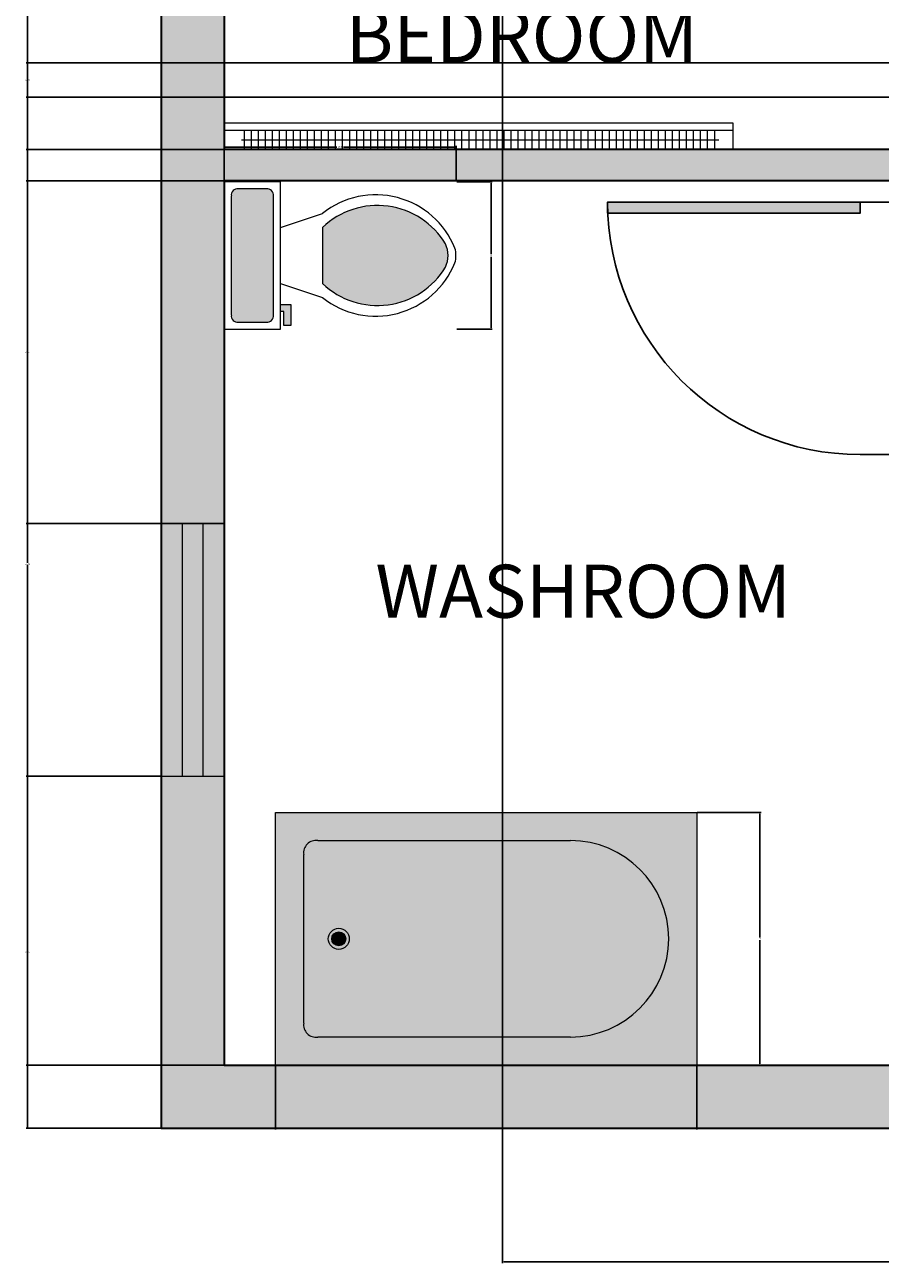
# Model space of a CAD drawing. Units: inches. Extents: x 857 to 1111, y 424 to 822.
# Tile 1 of 9: x 857 to 979, y 424 to 600. Entities that reach past the tile are written whole.
import ezdxf

# ---------------------------------------------------------------- set-up
doc = ezdxf.new("R2010")
doc.units = ezdxf.units.IN
for name, color, linetype, lineweight in [('A-ANNO-DIMS', 2, 'Continuous', 18), ('A-AREA-IDEN', 7, 'Continuous', 25), ('A-DETL', 7, 'Continuous', 18), ('A-DETL-PATT', 8, 'Continuous', 13), ('A-DOOR', 3, 'Continuous', 25), ('A-DOOR-PATT', 17, 'Continuous', 13), ('A-FLOR-FIXT', 8, 'Continuous', 20), ('A-FLOR-FIXT-PATT', 9, 'Continuous', 13), ('A-GLAZ', 4, 'Continuous', 18), ('A-GLAZ-PATT', 9, 'Continuous', 13), ('A-WALL', 7, 'Continuous', 35), ('A-WALL-PATT', 252, 'Continuous', 13)]:
    doc.layers.add(name, color=color, linetype=linetype, lineweight=lineweight)
doc.styles.get("Standard").update_dxf_attribs({"font": 'arial.ttf'})
doc.dimstyles.get("Standard").update_dxf_attribs({"dimtxt": 0.18, "dimasz": 0.18, "dimexe": 0.18, "dimexo": 0.0625, "dimgap": 0.09, "dimtad": 0, "dimtih": 1, "dimtoh": 1, "dimdec": 4, "dimzin": 0, "dimdsep": 46, "dimtxsty": 'Standard', "dimcen": 0.09, "dimadec": 0, "dimazin": 0, "dimtfac": 1, "dimtdec": 4, "dimtofl": 0, "dimtmove": 0, "dimatfit": 3, "dimfxl": 1, "dimtolj": 1, "dimtzin": 0, "dimarcsym": 0})

# ---------------------------------------------------------------- blocks, each defined once
blk = doc.blocks.new('Toilet - top')
for p, q in [((9.5, -6), (9.5, -2)), ((-10, -8.5), (-8, -8.5)), ((-10, -9.5), (-10, -8.5)), ((-8, -8.5), (-8, -8)), ((-7, -8), (-7, -9.5)), ((-4, -8), (-6, -14)), ((4, -8), (6, -14)), ((-7, -9.5), (-10, -9.5)), ((4, -14), (-4, -14))]:
    blk.add_line(p, q)
blk.add_lwpolyline([(10.5, -8), (10.5, 0), (-10.5, 0), (-10.5, -8)], close=True)
for points in [[(8.5, -1), (-8.5, -1)], [(-9.5, -2), (-9.5, -6)], [(-8.5, -7), (8.5, -7)]]:
    blk.add_lwpolyline(points)
for centre, radius, start, end in [((-8.62, -1.88), 0.884, 81.8699, 188.1301), ((8.62, -1.88), 0.884, 351.8699, 98.1301), ((-8.62, -6.12), 0.884, 171.8699, 278.1301), ((8.62, -6.12), 0.884, 261.8699, 8.1301), ((3.52, -21.58), 12.17, 141.4691, 247.9714), ((4.2, -21.82), 11.33, 136.3677, 238.9468), ((-3.52, -21.58), 12.17, 292.0284, 38.5307), ((-4.2, -21.82), 11.33, 301.053, 43.6321), ((0, -27.88), 4, 245.7318, 294.2682), ((0, -29), 4, 254.8605, 285.1395)]:
    blk.add_arc(centre, radius, start, end)
blk = doc.blocks.new('Bath Tub - 26 x 60 in.')
for p, q in [((9, -17), (9, -19)), ((8, -18), (10, -18))]:
    blk.add_line(p, q)
blk.add_lwpolyline([(0, -36), (0, 0), (60, 0), (60, -36)], close=True)
for points in [[(6, -4), (42, -4)], [(4, -30), (4, -6)], [(42, -32), (6, -32)]]:
    blk.add_lwpolyline(points)
for radius in [1.5, 1]:
    blk.add_circle((9, -18), radius)
for centre, radius, start, end in [((5.75, -5.75), 1.77, 81.8699, 188.1301), ((42, -18), 14, 270, 90), ((5.75, -30.25), 1.77, 171.8699, 278.1301)]:
    blk.add_arc(centre, radius, start, end)
blk = doc.blocks.new('*U16')
for p, q in [((0, 0), (0, -6)), ((-40, 0), (-40, -6))]:
    blk.add_line(p, q)
blk.add_lwpolyline([(0, 0), (0, 40), (-1.75, 40), (-1.75, 0)], close=True)
blk.add_arc((0, 0), 40, 90, 180)
blk = doc.blocks.new('WIN-36IN-9IN-WALL')
for p, q in [((3, 36), (3, 0)), ((6, 0), (6, 36))]:
    blk.add_line(p, q)
blk.add_lwpolyline([(0, 36), (0, 0), (9, 0), (9, 36)], close=True)
blk = doc.blocks.new('*D24')
at = {"layer": 'A-ANNO-DIMS', "color": 0, "lineweight": -2, "transparency": 16777216}
for p, q in [((885.14, 577.8), (885.14, 582.87)), ((885.32, 582.69), (901.19, 582.69)), ((918, 582.69), (902.13, 582.69)), ((918.18, 577.8), (918.18, 582.87))]:
    blk.add_line(p, q, dxfattribs=at)
at = {"layer": 'A-ANNO-DIMS', "color": 0, "transparency": 16777216}
for points in [[(885.32, 582.72), (885.32, 582.66), (885.14, 582.69)], [(918, 582.72), (918, 582.66), (918.18, 582.69)]]:
    blk.add_solid(points, dxfattribs=at)
at = {"layer": 'Defpoints', "color": 0, "transparency": 16777216}
for p in [(885.14, 582.69), (885.14, 577.73), (918.18, 577.73)]:
    blk.add_point(p, dxfattribs=at)
at = {"layer": 'A-ANNO-DIMS', "color": 0, "transparency": 16777216, "insert": (901.66, 582.69), "char_height": 0.18, "attachment_point": 5}
blk.add_mtext('\\A1;WC 33', dxfattribs=at)
blk = doc.blocks.new('*D25')
at = {"layer": 'A-ANNO-DIMS', "color": 0, "lineweight": -2, "transparency": 16777216}
for p, q in [((918.25, 577.73), (923.32, 577.73)), ((923.14, 577.55), (923.14, 567.42)), ((923.14, 556.91), (923.14, 567.05)), ((918.25, 556.73), (923.32, 556.73))]:
    blk.add_line(p, q, dxfattribs=at)
at = {"layer": 'A-ANNO-DIMS', "color": 0, "transparency": 16777216}
for points in [[(923.11, 577.55), (923.17, 577.55), (923.14, 577.73)], [(923.11, 556.91), (923.17, 556.91), (923.14, 556.73)]]:
    blk.add_solid(points, dxfattribs=at)
at = {"layer": 'Defpoints', "color": 0, "transparency": 16777216}
for p in [(918.18, 577.73), (923.14, 577.73), (918.18, 556.73)]:
    blk.add_point(p, dxfattribs=at)
at = {"layer": 'A-ANNO-DIMS', "color": 0, "transparency": 16777216, "insert": (923.14, 567.23), "char_height": 0.18, "attachment_point": 5}
blk.add_mtext('\\A1;21', dxfattribs=at)
blk = doc.blocks.new('*D26')
at = {"layer": 'A-ANNO-DIMS', "color": 0, "lineweight": -2, "transparency": 16777216}
for p, q in [((892.45, 451.79), (892.45, 442.68)), ((952.45, 451.79), (952.45, 442.68)), ((892.63, 442.86), (921.94, 442.86)), ((952.27, 442.86), (922.96, 442.86))]:
    blk.add_line(p, q, dxfattribs=at)
at = {"layer": 'A-ANNO-DIMS', "color": 0, "transparency": 16777216}
for points in [[(892.63, 442.89), (892.63, 442.83), (892.45, 442.86)], [(952.27, 442.89), (952.27, 442.83), (952.45, 442.86)]]:
    blk.add_solid(points, dxfattribs=at)
at = {"layer": 'Defpoints', "color": 0, "transparency": 16777216}
for p in [(892.45, 451.86), (952.45, 451.86), (952.45, 442.86)]:
    blk.add_point(p, dxfattribs=at)
at = {"layer": 'A-ANNO-DIMS', "color": 0, "transparency": 16777216, "insert": (922.45, 442.86), "char_height": 0.18, "attachment_point": 5}
blk.add_mtext('\\A1;TUB 60', dxfattribs=at)
blk = doc.blocks.new('*D27')
at = {"layer": 'A-ANNO-DIMS', "color": 0, "lineweight": -2, "transparency": 16777216}
for p, q in [((952.51, 487.86), (961.63, 487.86)), ((961.45, 487.68), (961.45, 470.04)), ((961.45, 452.04), (961.45, 469.67)), ((952.51, 451.86), (961.63, 451.86))]:
    blk.add_line(p, q, dxfattribs=at)
at = {"layer": 'A-ANNO-DIMS', "color": 0, "transparency": 16777216}
for points in [[(961.42, 487.68), (961.48, 487.68), (961.45, 487.86)], [(961.42, 452.04), (961.48, 452.04), (961.45, 451.86)]]:
    blk.add_solid(points, dxfattribs=at)
at = {"layer": 'Defpoints', "color": 0, "transparency": 16777216}
for p in [(952.45, 487.86), (961.45, 487.86), (952.45, 451.86)]:
    blk.add_point(p, dxfattribs=at)
at = {"layer": 'A-ANNO-DIMS', "color": 0, "transparency": 16777216, "insert": (961.45, 469.86), "char_height": 0.18, "attachment_point": 5}
blk.add_mtext('\\A1;36', dxfattribs=at)
blk = doc.blocks.new('*D48')
at = {"layer": 'A-ANNO-DIMS', "color": 0, "lineweight": -2, "transparency": 16777216}
for p, q in [((885.14, 582.42), (885.14, 822.09)), ((885.32, 821.91), (935, 821.91)), ((985.46, 821.91), (935.77, 821.91)), ((985.64, 582.42), (985.64, 822.09))]:
    blk.add_line(p, q, dxfattribs=at)
at = {"layer": 'A-ANNO-DIMS', "color": 0, "transparency": 16777216}
for points in [[(885.32, 821.94), (885.32, 821.88), (885.14, 821.91)], [(985.46, 821.94), (985.46, 821.88), (985.64, 821.91)]]:
    blk.add_solid(points, dxfattribs=at)
at = {"layer": 'Defpoints', "color": 0, "transparency": 16777216}
for p in [(985.64, 821.91), (885.14, 582.36), (985.64, 582.36)]:
    blk.add_point(p, dxfattribs=at)
at = {"layer": 'A-ANNO-DIMS', "color": 0, "transparency": 16777216, "insert": (935.39, 821.91), "char_height": 0.18, "attachment_point": 5}
blk.add_mtext('\\A1;100.5', dxfattribs=at)
blk = doc.blocks.new('*D53')
at = {"layer": 'A-ANNO-DIMS', "color": 0, "lineweight": -2, "transparency": 16777216}
for p, q in [((1035.07, 594.69), (856.91, 594.69)), ((857.09, 594.51), (857.09, 523.46)), ((857.09, 452.04), (857.09, 523.09)), ((1035.07, 451.86), (856.91, 451.86))]:
    blk.add_line(p, q, dxfattribs=at)
at = {"layer": 'A-ANNO-DIMS', "color": 0, "transparency": 16777216}
for points in [[(857.06, 594.51), (857.12, 594.51), (857.09, 594.69)], [(857.06, 452.04), (857.12, 452.04), (857.09, 451.86)]]:
    blk.add_solid(points, dxfattribs=at)
at = {"layer": 'Defpoints', "color": 0, "transparency": 16777216}
for p in [(857.09, 594.69), (1035.14, 594.69), (1035.14, 451.86)]:
    blk.add_point(p, dxfattribs=at)
at = {"layer": 'A-ANNO-DIMS', "color": 0, "transparency": 16777216, "insert": (857.09, 523.28), "char_height": 0.18, "attachment_point": 5}
blk.add_mtext('\\A1;142.84', dxfattribs=at)
blk = doc.blocks.new('*D56')
at = {"layer": 'A-ANNO-DIMS', "color": 0, "lineweight": -2, "transparency": 16777216}
for p, q in [((924.77, 717.29), (924.77, 423.63)), ((1053.97, 717.29), (1053.97, 423.63)), ((924.95, 423.81), (988.99, 423.81)), ((1053.79, 423.81), (989.75, 423.81))]:
    blk.add_line(p, q, dxfattribs=at)
at = {"layer": 'A-ANNO-DIMS', "color": 0, "transparency": 16777216}
for points in [[(924.95, 423.84), (924.95, 423.78), (924.77, 423.81)], [(1053.79, 423.84), (1053.79, 423.78), (1053.97, 423.81)]]:
    blk.add_solid(points, dxfattribs=at)
at = {"layer": 'Defpoints', "color": 0, "transparency": 16777216}
for p in [(924.77, 717.36), (1053.97, 717.36), (1053.97, 423.81)]:
    blk.add_point(p, dxfattribs=at)
at = {"layer": 'A-ANNO-DIMS', "color": 0, "transparency": 16777216, "insert": (989.37, 423.81), "char_height": 0.18, "attachment_point": 5}
blk.add_mtext('\\A1;129.2', dxfattribs=at)
blk = doc.blocks.new('*D57')
at = {"layer": 'A-ANNO-DIMS', "color": 0, "lineweight": -2, "transparency": 16777216}
for p, q in [((876.07, 493.04), (856.91, 493.04)), ((857.09, 492.86), (857.09, 468.13)), ((857.09, 443.04), (857.09, 467.76)), ((876.07, 442.86), (856.91, 442.86))]:
    blk.add_line(p, q, dxfattribs=at)
at = {"layer": 'A-ANNO-DIMS', "color": 0, "transparency": 16777216}
for points in [[(857.06, 492.86), (857.12, 492.86), (857.09, 493.04)], [(857.06, 443.04), (857.12, 443.04), (857.09, 442.86)]]:
    blk.add_solid(points, dxfattribs=at)
at = {"layer": 'Defpoints', "color": 0, "transparency": 16777216}
for p in [(857.09, 493.04), (876.14, 493.04), (876.14, 442.86)]:
    blk.add_point(p, dxfattribs=at)
at = {"layer": 'A-ANNO-DIMS', "color": 0, "transparency": 16777216, "insert": (857.09, 467.95), "char_height": 0.18, "attachment_point": 5}
blk.add_mtext('\\A1;50.18', dxfattribs=at)
blk = doc.blocks.new('*D58')
at = {"layer": 'A-ANNO-DIMS', "color": 0, "lineweight": -2, "transparency": 16777216}
for p, q in [((885.07, 577.86), (856.91, 577.86)), ((857.09, 577.68), (857.09, 553.63)), ((857.09, 529.22), (857.09, 553.26)), ((885.07, 529.04), (856.91, 529.04))]:
    blk.add_line(p, q, dxfattribs=at)
at = {"layer": 'A-ANNO-DIMS', "color": 0, "transparency": 16777216}
for points in [[(857.06, 577.68), (857.12, 577.68), (857.09, 577.86)], [(857.06, 529.22), (857.12, 529.22), (857.09, 529.04)]]:
    blk.add_solid(points, dxfattribs=at)
at = {"layer": 'Defpoints', "color": 0, "transparency": 16777216}
for p in [(857.09, 577.86), (885.14, 577.86), (885.14, 529.04)]:
    blk.add_point(p, dxfattribs=at)
at = {"layer": 'A-ANNO-DIMS', "color": 0, "transparency": 16777216, "insert": (857.09, 553.45), "char_height": 0.18, "attachment_point": 5}
blk.add_mtext('\\A1;48.82', dxfattribs=at)
blk = doc.blocks.new('*D59')
at = {"layer": 'A-ANNO-DIMS', "color": 0, "lineweight": -2, "transparency": 16777216}
for p, q in [((885.07, 628.69), (856.91, 628.69)), ((857.09, 628.51), (857.09, 605.7)), ((857.09, 582.54), (857.09, 605.34)), ((885.07, 582.36), (856.91, 582.36))]:
    blk.add_line(p, q, dxfattribs=at)
at = {"layer": 'A-ANNO-DIMS', "color": 0, "transparency": 16777216}
for points in [[(857.06, 628.51), (857.12, 628.51), (857.09, 628.69)], [(857.06, 582.54), (857.12, 582.54), (857.09, 582.36)]]:
    blk.add_solid(points, dxfattribs=at)
at = {"layer": 'Defpoints', "color": 0, "transparency": 16777216}
for p in [(857.09, 628.69), (885.14, 628.69), (885.14, 582.36)]:
    blk.add_point(p, dxfattribs=at)
at = {"layer": 'A-ANNO-DIMS', "color": 0, "transparency": 16777216, "insert": (857.09, 605.52), "char_height": 0.18, "attachment_point": 5}
blk.add_mtext('\\A1;46.33', dxfattribs=at)
blk = doc.blocks.new('*D60')
at = {"layer": 'A-ANNO-DIMS', "color": 0, "lineweight": -2, "transparency": 16777216}
for p, q in [((1083.07, 594.69), (856.91, 594.69)), ((857.09, 594.51), (857.09, 592.43)), ((857.09, 589.98), (857.09, 592.07)), ((1083.07, 589.8), (856.91, 589.8))]:
    blk.add_line(p, q, dxfattribs=at)
at = {"layer": 'A-ANNO-DIMS', "color": 0, "transparency": 16777216}
for points in [[(857.06, 594.51), (857.12, 594.51), (857.09, 594.69)], [(857.06, 589.98), (857.12, 589.98), (857.09, 589.8)]]:
    blk.add_solid(points, dxfattribs=at)
at = {"layer": 'Defpoints', "color": 0, "transparency": 16777216}
for p in [(857.09, 594.69), (1083.14, 594.69), (1083.14, 589.8)]:
    blk.add_point(p, dxfattribs=at)
at = {"layer": 'A-ANNO-DIMS', "color": 0, "transparency": 16777216, "insert": (857.09, 592.25), "char_height": 0.18, "attachment_point": 5}
blk.add_mtext('\\A1;4.891', dxfattribs=at)

msp = doc.modelspace()

# ---------------------------------------------------------------- hatches: boundary and pattern name
at = {"layer": 'A-DETL-PATT'}
h = msp.add_hatch(dxfattribs=at)
h.set_pattern_fill('ANSI31', color=256, scale=0.314961, angle=45, style=0)
h.paths.add_polyline_path([(887.6043, 582.3567), (955.6043, 582.3567), (955.6043, 585.1154), (887.6043, 585.1154)])
at = {"layer": 'A-DOOR-PATT'}
h = msp.add_hatch(color=256, dxfattribs=at)
h.dxf.hatch_style = 1
h.paths.add_polyline_path([(975.7391, 574.8417), (939.754, 574.8417, 0.01094143), (939.7885, 573.2674), (975.7391, 573.2674)])
h.paths.add_polyline_path([(985.6369, 577.8567), (981.1369, 577.8567), (981.1369, 574.8567), (985.6369, 574.8567)])
h.paths.add_polyline_path([(985.6369, 538.8567), (981.1369, 538.8567), (981.1369, 535.8567), (985.6369, 535.8567)])
h.paths.add_polyline_path([(993.2112, 493.205, 0.01094143), (991.6369, 493.2395), (991.6369, 457.2544), (993.2112, 457.2544)])
at = {"layer": 'A-FLOR-FIXT-PATT'}
h = msp.add_hatch(color=256, dxfattribs=at)
h.dxf.hatch_style = 1
h.paths.add_polyline_path([(892.1369, 575.7347, 0.50000012), (891.1369, 576.7347), (887.1369, 576.7347, 0.50000012), (886.1369, 575.7347), (886.1369, 558.7347, 0.50000012), (887.1369, 557.7347), (891.1369, 557.7347, 0.50000012), (892.1369, 558.7347)])
h.paths.add_polyline_path([(916.6599, 568.8788, 0.4800795), (899.1369, 571.2348), (899.1369, 563.2348, 0.48007965), (916.6599, 565.5907, 0.21500378)])
h.paths.add_polyline_path([(894.6369, 560.2347), (893.1369, 560.2347), (893.1369, 559.2347), (893.6369, 559.2347), (893.6369, 557.2347), (894.6369, 557.2347)])
h = msp.add_hatch(color=256, dxfattribs=at)
h.dxf.hatch_style = 1
h.paths.add_polyline_path([(952.4491, 487.8567), (892.4491, 487.8567), (892.4491, 451.8567), (952.4491, 451.8567)])
h.paths.add_polyline_path([(898.4491, 483.8567), (934.4491, 483.8567, -1), (934.4491, 455.8567), (898.4491, 455.8567, -0.50000012), (896.4491, 457.8567), (896.4491, 481.8567, -0.50000012)], flags=16)
h.paths.add_polyline_path([(902.9491, 469.8567, -1), (899.9491, 469.8567, -1)], flags=0)
h.paths.add_polyline_path([(902.4491, 469.8567, -1), (900.4491, 469.8567, -1)], flags=0)
h = msp.add_hatch(color=256, dxfattribs=at)
h.dxf.hatch_style = 1
h.paths.add_polyline_path([(934.4491, 483.8567), (898.4491, 483.8567, 0.50000012), (896.4491, 481.8567), (896.4491, 457.8567, 0.50000012), (898.4491, 455.8567), (934.4491, 455.8567, 1)])
h.paths.add_polyline_path([(899.9491, 469.8567, -1), (902.9491, 469.8567, -1)], flags=16)
h.paths.add_polyline_path([(900.4491, 469.8567, -1), (902.4491, 469.8567, -1)], flags=0)
h = msp.add_hatch(color=256, dxfattribs=at)
h.dxf.hatch_style = 1
h.paths.add_polyline_path([(902.4491, 469.8567), (901.4491, 469.8567), (901.4491, 468.8567, 0.41421356)], flags=0)
h.paths.add_polyline_path([(901.4491, 470.8567), (901.4491, 469.8567), (902.4491, 469.8567, 0.41421356)], flags=0)
h.paths.add_polyline_path([(901.4491, 470.8567, 0.41421356), (900.4491, 469.8567), (901.4491, 469.8567)], flags=0)
h.paths.add_polyline_path([(901.4491, 469.8567), (900.4491, 469.8567, 0.41421356), (901.4491, 468.8567)], flags=0)
h.paths.add_polyline_path([(902.9491, 469.8567, 1), (899.9491, 469.8567, 1)])
h.paths.add_polyline_path([(900.4491, 469.8567, -1), (902.4491, 469.8567, -1)], flags=16)
h = msp.add_hatch(color=256, dxfattribs=at)
h.dxf.hatch_style = 1
h.paths.add_polyline_path([(901.4491, 470.8567, 0.41421356), (900.4491, 469.8567), (901.4491, 469.8567)])
h.paths.add_polyline_path([(901.4491, 470.8567), (901.4491, 469.8567), (902.4491, 469.8567, 0.41421356)])
h.paths.add_polyline_path([(902.4491, 469.8567), (901.4491, 469.8567), (901.4491, 468.8567, 0.41421356)])
h.paths.add_polyline_path([(901.4491, 469.8567), (900.4491, 469.8567, 0.41421356), (901.4491, 468.8567)])
at = {"layer": 'A-GLAZ-PATT'}
h = msp.add_hatch(color=256, dxfattribs=at)
h.dxf.hatch_style = 1
h.set_gradient(color1=(0, 0, 255), color2=(255, 255, 0), name='SPHERICAL')
h.paths.add_polyline_path([(885.1369, 529.0363), (882.1369, 529.0363), (882.1369, 493.0363), (885.1369, 493.0363)])
h.paths.add_polyline_path([(882.1369, 529.0363), (879.1369, 529.0363), (879.1369, 493.0363), (882.1369, 493.0363)])
h.paths.add_polyline_path([(879.1369, 529.0363), (876.1369, 529.0363), (876.1369, 493.0363), (879.1369, 493.0363)])
at = {"layer": 'A-WALL-PATT'}
h = msp.add_hatch(color=256, dxfattribs=at)
h.dxf.hatch_style = 1
h.paths.add_polyline_path([(924.7696, 721.8567), (885.1369, 721.8567), (885.1369, 793.8567), (1083.1369, 793.8567), (1083.1369, 721.8567), (1053.9717, 721.8567), (1053.9717, 717.3567), (1083.1369, 717.3567), (1083.1369, 706.6069), (1092.1369, 706.6069), (1092.1369, 802.8567), (876.1369, 802.8567), (876.1369, 664.6868), (885.1369, 664.6868), (885.1369, 717.3567), (924.7696, 717.3567)])
h.paths.add_polyline_path([(985.6369, 582.3567), (885.1369, 582.3567), (885.1369, 585.1154), (885.1369, 628.6868), (876.1369, 628.6868), (876.1369, 529.0363), (885.1369, 529.0363), (885.1369, 577.8567), (981.1369, 577.8567), (985.6369, 577.8567)])
h.paths.add_polyline_path([(885.1369, 493.0363), (876.1369, 493.0363), (876.1369, 442.8567), (991.6369, 442.8567), (991.6369, 451.8567), (985.6369, 451.8567), (985.6369, 535.8567), (981.1369, 535.8567), (981.1369, 451.8567), (885.1369, 451.8567)])
h.paths.add_polyline_path([(1092.1369, 553.8025), (1083.1369, 553.8025), (1083.1369, 451.8567), (1030.6369, 451.8567), (1027.6369, 451.8567), (1027.6369, 442.8567), (1092.1369, 442.8567)])
h.paths.add_polyline_path([(1092.1369, 670.6069), (1083.1369, 670.6069), (1083.1369, 662.5384, -0.02676862), (1083.1369, 657.4501), (1083.1369, 589.8025), (1092.1369, 589.8025)])

# ---------------------------------------------------------------- linework, layer by layer
at = {"layer": 'A-DETL'}
for p, q in [((885.1369, 586.1154), (957.6043, 586.1154)), ((957.6043, 586.1154), (957.6043, 582.3567)), ((885.1369, 585.1154), (957.6043, 585.1154)), ((885.1369, 582.3567), (885.1369, 585.1154)), ((887.6043, 583.736), (955.6043, 583.736)), ((957.6043, 582.3567), (885.1369, 582.3567))]:
    msp.add_line(p, q, dxfattribs=at)
at = {"layer": 'A-WALL'}
for p, q in [((885.1369, 717.3567), (885.1369, 582.3567)), ((985.6369, 582.3567), (885.1369, 582.3567)), ((981.1369, 577.8567), (885.1369, 577.8567)), ((885.1369, 577.8567), (885.1369, 451.8567)), ((885.1369, 451.8567), (981.1369, 451.8567))]:
    msp.add_line(p, q, dxfattribs=at)
msp.add_lwpolyline([(1027.6369, 442.8567), (1092.1369, 442.8567), (1092.1369, 802.8567), (876.1369, 802.8567), (876.1369, 442.8567), (991.6369, 442.8567)], dxfattribs=at)

# ---------------------------------------------------------------- block references
at = {"layer": 'A-DOOR', "xscale": 0.8996270808511326, "yscale": 0.8996270808511326, "zscale": 0.8996270808511326, "rotation": 90}
msp.add_blockref('*U16', (975.7391, 574.8417), dxfattribs=at)
at = {"layer": 'A-FLOR-FIXT', "rotation": 90}
msp.add_blockref('Toilet - top', (885.1369, 567.2347), dxfattribs=at)
at = {"layer": 'A-FLOR-FIXT'}
msp.add_blockref('Bath Tub - 26 x 60 in.', (892.4491, 487.8567), dxfattribs=at)
at = {"layer": 'A-GLAZ'}
msp.add_blockref('WIN-36IN-9IN-WALL', (876.1369, 493.0363), dxfattribs=at)

# ---------------------------------------------------------------- texts
at = {"layer": 'A-AREA-IDEN'}
for s, p in [('BEDROOM ', (902.4461, 594.7313)), ('WASHROOM ', (906.6739, 515.6066))]:
    msp.add_text(s, height=7.55928, dxfattribs=at).set_placement(p)

# ---------------------------------------------------------------- dimensions: what is measured, and where the dimension line sits
at = {"layer": 'A-ANNO-DIMS'}
for base, p1, p2, picture, middle in [((985.6369, 821.9067), (885.1369, 582.3567), (985.6369, 582.3567), '*D48', (935.3869, 821.9067)), ((1053.9717, 423.8067), (924.7696, 717.3567), (1053.9717, 717.3567), '*D56', (989.3707, 423.8067))]:
    dim = msp.add_linear_dim(base=base, p1=p1, p2=p2, dimstyle='Standard', override={"dimdec": 1, "dimlfac": 1, "dimrnd": 0, "dimzin": 0, "dimdsep": 46, "dimlunit": 2}, dxfattribs=at)
    dim.commit()
    dim.dimension.update_dxf_attribs({"geometry": picture, "text_midpoint": middle})
for base, p1, p2, override, picture, middle in [((857.0869, 628.6868), (885.1369, 582.3567), (885.1369, 628.6868), {"dimdec": 2, "dimlfac": 1, "dimrnd": 0, "dimzin": 0, "dimdsep": 46, "dimlunit": 2}, '*D59', (857.0869, 605.5217)), ((857.0869, 594.6935), (1035.1369, 451.8567), (1035.1369, 594.6935), {"dimdec": 2, "dimlfac": 1, "dimrnd": 0, "dimzin": 0, "dimdsep": 46, "dimlunit": 2}, '*D53', (857.0869, 523.2751)), ((857.0869, 594.6935), (1083.1369, 589.8025), (1083.1369, 594.6935), {"dimdec": 3, "dimlfac": 1, "dimrnd": 0, "dimzin": 0, "dimdsep": 46, "dimlunit": 2}, '*D60', (857.0869, 592.248)), ((857.0869, 577.8567), (885.1369, 529.0363), (885.1369, 577.8567), {"dimdec": 2, "dimlfac": 1, "dimrnd": 0, "dimzin": 0, "dimdsep": 46, "dimlunit": 2}, '*D58', (857.0869, 553.4465)), ((923.1401, 577.7347), (918.1831, 556.7347), (918.1831, 577.7347), {"dimdec": 0, "dimlfac": 1, "dimrnd": 0, "dimzin": 0, "dimdsep": 46, "dimlunit": 2}, '*D25', (923.1401, 567.2347)), ((857.0869, 493.0363), (876.1369, 442.8567), (876.1369, 493.0363), {"dimdec": 2, "dimlfac": 1, "dimrnd": 0, "dimzin": 0, "dimdsep": 46, "dimlunit": 2}, '*D57', (857.0869, 467.9465)), ((961.4491, 487.8567), (952.4491, 451.8567), (952.4491, 487.8567), {"dimdec": 0, "dimlfac": 1, "dimrnd": 0, "dimzin": 0, "dimdsep": 46, "dimlunit": 2}, '*D27', (961.4491, 469.8567))]:
    dim = msp.add_linear_dim(base=base, p1=p1, p2=p2, angle=90, dimstyle='Standard', override=override, dxfattribs=at)
    dim.commit()
    dim.dimension.update_dxf_attribs({"geometry": picture, "text_midpoint": middle})
dim = msp.add_linear_dim(base=(885.1369, 582.6917), p1=(918.1831, 577.7347), p2=(885.1369, 577.7347), angle=180, text='WC <>', dimstyle='Standard', override={"dimdec": 0, "dimlfac": 1, "dimrnd": 0, "dimzin": 0, "dimdsep": 46, "dimlunit": 2}, dxfattribs=at)
dim.commit()
dim.dimension.update_dxf_attribs({"geometry": '*D24', "text_midpoint": (901.66, 582.6917)})
dim = msp.add_linear_dim(base=(952.4491, 442.8567), p1=(892.4491, 451.8567), p2=(952.4491, 451.8567), text='TUB <>', dimstyle='Standard', override={"dimdec": 0, "dimlfac": 1, "dimrnd": 0, "dimzin": 0, "dimdsep": 46, "dimlunit": 2}, dxfattribs=at)
dim.commit()
dim.dimension.update_dxf_attribs({"geometry": '*D26', "text_midpoint": (922.4491, 442.8567)})

doc.saveas('drawing.dxf')
